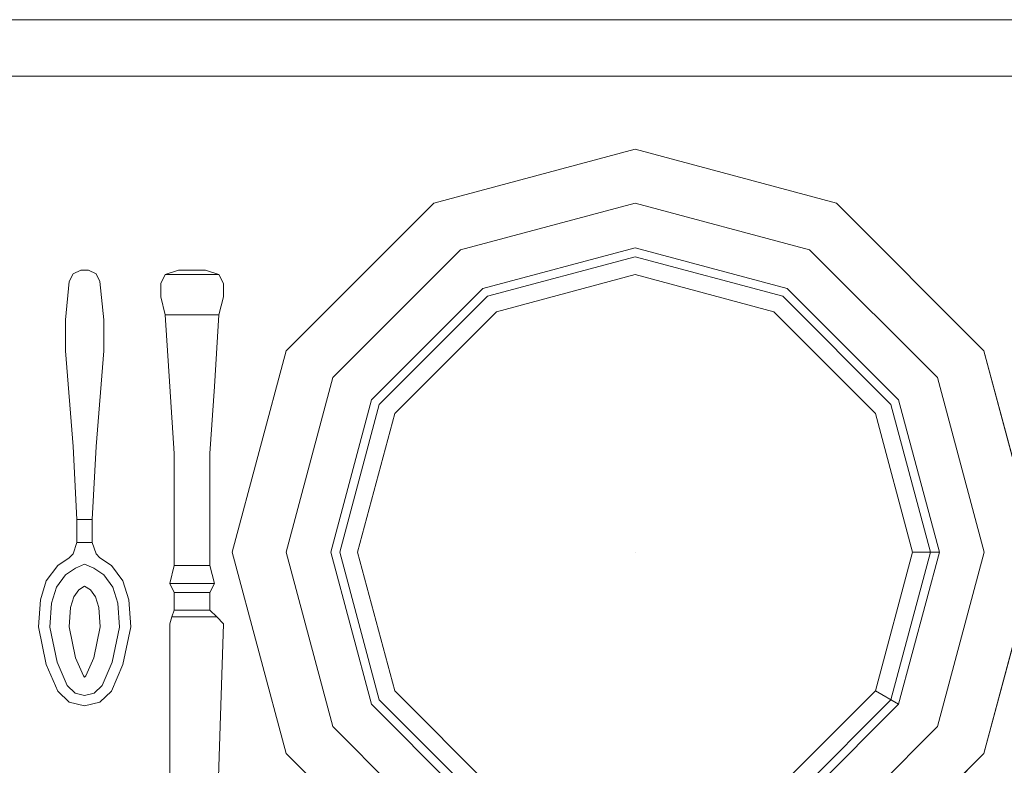
# Model space of a CAD drawing. Units: inches. Extents: x 375 to 1122, y 27 to 1069.
# Tile 54 of 155: x 717.62 to 731.16, y 314.24 to 324.5. Entities that reach past the tile are written whole.
import ezdxf

# ---------------------------------------------------------------- set-up
doc = ezdxf.new("R2010")
doc.units = ezdxf.units.IN
doc.layers.add('Furniture', color=30, linetype='Continuous', lineweight=18)

# ---------------------------------------------------------------- blocks, each defined once
blk = doc.blocks.new('A$C403C54AD')
for p, q in [((0.54488, 0.79569, -0.0006), (0.54488, 1.26108, -0.0006)), ((0.56427, 0.79569, -0.0006), (0.56427, 1.26108, -0.0006))]:
    blk.add_line(p, q)
at = {"linetype": 'ByBlock'}
for points, invisible_edges in [([(0.72796, 1.16691, -0.0197), (0.72796, 1.14844, -0.0197), (0.66793, 1.13235, -0.0197), (0.6587, 1.14835, -0.0197)], 5), ([(0.72796, 1.13305, -0.03355), (0.72796, 1.16691, -0.02431), (0.6587, 1.14835, -0.02431), (0.67563, 1.11902, -0.03355)], 5), ([(0.79723, 1.14835, -0.0197), (0.78799, 1.13235, -0.0197), (0.72796, 1.14844, -0.0197), (0.72796, 1.16691, -0.0197)], 5), ([(0.7803, 1.11902, -0.03355), (0.79723, 1.14835, -0.02431), (0.72796, 1.16691, -0.02431), (0.72796, 1.13305, -0.03355)], 5), ([(0.6587, 1.14835, -0.0197), (0.66793, 1.13235, -0.0197), (0.62399, 1.08841, -0.0197), (0.60799, 1.09765, -0.0197)], 5), ([(0.67563, 1.11902, -0.03355), (0.6587, 1.14835, -0.02431), (0.60799, 1.09765, -0.02431), (0.63732, 1.08071, -0.03355)], 5), ([(0.72796, 1.14844, -0.0197), (0.72796, 1.12997, -0.02585), (0.67717, 1.11636, -0.02585), (0.66793, 1.13235, -0.0197)], 5), ([(0.78799, 1.13235, -0.0197), (0.77876, 1.11636, -0.02585), (0.72796, 1.12997, -0.02585), (0.72796, 1.14844, -0.0197)], 5), ([(0.81861, 1.08071, -0.03355), (0.84793, 1.09765, -0.02431), (0.79723, 1.14835, -0.02431), (0.7803, 1.11902, -0.03355)], 5), ([(0.84793, 1.09765, -0.0197), (0.83194, 1.08841, -0.0197), (0.78799, 1.13235, -0.0197), (0.79723, 1.14835, -0.0197)], 5), ([(0.66793, 1.13235, -0.0197), (0.67717, 1.11636, -0.02585), (0.63999, 1.07918, -0.02585), (0.62399, 1.08841, -0.0197)], 5), ([(0.72796, 1.12381, -0.04278), (0.72796, 1.13305, -0.03355), (0.67563, 1.11902, -0.03355), (0.68025, 1.11103, -0.04278)], 4), ([(0.83194, 1.08841, -0.0197), (0.81594, 1.07918, -0.02585), (0.77876, 1.11636, -0.02585), (0.78799, 1.13235, -0.0197)], 5), ([(0.72796, 1.12997, -0.02585), (0.72796, 1.02838, -0.02585), (0.72796, 1.02838, -0.02585), (0.67717, 1.11636, -0.02585)], 5), ([(0.77876, 1.11636, -0.02585), (0.72796, 1.02838, -0.02585), (0.72796, 1.02838, -0.02585), (0.72796, 1.12997, -0.02585)], 5), ([(0.68025, 1.11103, -0.04278), (0.67563, 1.11902, -0.03355), (0.63732, 1.08071, -0.03355), (0.64532, 1.0761, -0.04278)], 5), ([(0.81061, 1.0761, -0.04278), (0.81861, 1.08071, -0.03355), (0.7803, 1.11902, -0.03355), (0.77568, 1.11103, -0.04278)], 1), ([(0.67717, 1.11636, -0.02585), (0.72796, 1.02838, -0.02585), (0.72796, 1.02838, -0.02585), (0.63999, 1.07918, -0.02585)], 5), ([(0.81594, 1.07918, -0.02585), (0.72796, 1.02838, -0.02585), (0.72796, 1.02838, -0.02585), (0.77876, 1.11636, -0.02585)], 5), ([(0.60799, 1.09765, -0.0197), (0.62399, 1.08841, -0.0197), (0.60791, 1.02838, -0.0197), (0.58944, 1.02838, -0.0197)], 5), ([(0.63732, 1.08071, -0.03355), (0.60799, 1.09765, -0.02431), (0.58944, 1.02838, -0.02431), (0.6233, 1.02838, -0.03355)], 5), ([(0.62399, 1.08841, -0.0197), (0.63999, 1.07918, -0.02585), (0.62638, 1.02838, -0.02585), (0.60791, 1.02838, -0.0197)], 5), ([(0.64532, 1.0761, -0.04278), (0.63732, 1.08071, -0.03355), (0.6233, 1.02838, -0.03355), (0.63253, 1.02838, -0.04278)], 5), ([(0.63999, 1.07918, -0.02585), (0.72796, 1.02838, -0.02585), (0.72796, 1.02838, -0.02585), (0.62638, 1.02838, -0.02585)], 5), ([(0.82955, 1.02838, -0.02585), (0.72796, 1.02838, -0.02585), (0.72796, 1.02838, -0.02585), (0.81594, 1.07918, -0.02585)], 5), ([(0.58944, 1.02838, -0.0197), (0.60791, 1.02838, -0.0197), (0.62399, 0.96835, -0.0197), (0.60799, 0.95912, -0.0197)], 5), ([(0.6233, 1.02838, -0.03355), (0.58944, 1.02838, -0.02431), (0.60799, 0.95912, -0.02431), (0.63732, 0.97605, -0.03355)], 5), ([(0.60791, 1.02838, -0.0197), (0.62638, 1.02838, -0.02585), (0.63999, 0.97759, -0.02585), (0.62399, 0.96835, -0.0197)], 5), ([(0.63253, 1.02838, -0.04278), (0.6233, 1.02838, -0.03355), (0.63732, 0.97605, -0.03355), (0.64532, 0.98067, -0.04278)], 5), ([(0.62638, 1.02838, -0.02585), (0.72796, 1.02838, -0.02585), (0.72796, 1.02838, -0.02585), (0.63999, 0.97759, -0.02585)], 5), ([(0.63999, 0.97759, -0.02585), (0.72796, 1.02838, -0.02585), (0.72796, 1.02838, -0.02585), (0.67717, 0.94041, -0.02585)], 5), ([(0.67717, 0.94041, -0.02585), (0.72796, 1.02838, -0.02585), (0.72796, 1.02838, -0.02585), (0.72796, 0.9268, -0.02585)], 5), ([(0.81594, 0.97759, -0.02585), (0.72796, 1.02838, -0.02585), (0.72796, 1.02838, -0.02585), (0.82955, 1.02838, -0.02585)], 5), ([(0.77876, 0.94041, -0.02585), (0.72796, 1.02838, -0.02585), (0.72796, 1.02838, -0.02585), (0.81594, 0.97759, -0.02585)], 5), ([(0.72796, 0.9268, -0.02585), (0.72796, 1.02838, -0.02585), (0.72796, 1.02838, -0.02585), (0.77876, 0.94041, -0.02585)], 5), ([(0.64532, 0.98067, -0.04278), (0.63732, 0.97605, -0.03355), (0.67563, 0.93774, -0.03355), (0.68025, 0.94574, -0.04278)], 5), ([(0.77568, 0.94574, -0.04278), (0.7803, 0.93774, -0.03355), (0.81861, 0.97605, -0.03355), (0.81061, 0.98067, -0.04278)], 5), ([(0.63732, 0.97605, -0.03355), (0.60799, 0.95912, -0.02431), (0.6587, 0.90841, -0.02431), (0.67563, 0.93774, -0.03355)], 5), ([(0.62399, 0.96835, -0.0197), (0.63999, 0.97759, -0.02585), (0.67717, 0.94041, -0.02585), (0.66793, 0.92441, -0.0197)], 5), ([(0.78799, 0.92441, -0.0197), (0.77876, 0.94041, -0.02585), (0.81594, 0.97759, -0.02585), (0.83194, 0.96835, -0.0197)], 5), ([(0.7803, 0.93774, -0.03355), (0.79723, 0.90841, -0.02431), (0.84793, 0.95912, -0.02431), (0.81861, 0.97605, -0.03355)], 5), ([(0.60799, 0.95912, -0.0197), (0.62399, 0.96835, -0.0197), (0.66793, 0.92441, -0.0197), (0.6587, 0.90841, -0.0197)], 5), ([(0.79723, 0.90841, -0.0197), (0.78799, 0.92441, -0.0197), (0.83194, 0.96835, -0.0197), (0.84793, 0.95912, -0.0197)], 5), ([(0.68025, 0.94574, -0.04278), (0.67563, 0.93774, -0.03355), (0.72796, 0.92372, -0.03355), (0.72796, 0.93295, -0.04278)], 5), ([(0.72796, 0.93295, -0.04278), (0.72796, 0.92372, -0.03355), (0.7803, 0.93774, -0.03355), (0.77568, 0.94574, -0.04278)], 5), ([(0.66793, 0.92441, -0.0197), (0.67717, 0.94041, -0.02585), (0.72796, 0.9268, -0.02585), (0.72796, 0.90833, -0.0197)], 5), ([(0.72796, 0.90833, -0.0197), (0.72796, 0.9268, -0.02585), (0.77876, 0.94041, -0.02585), (0.78799, 0.92441, -0.0197)], 5), ([(0.67563, 0.93774, -0.03355), (0.6587, 0.90841, -0.02431), (0.72796, 0.88985, -0.02431), (0.72796, 0.92372, -0.03355)], 5), ([(0.72796, 0.92372, -0.03355), (0.72796, 0.88985, -0.02431), (0.79723, 0.90841, -0.02431), (0.7803, 0.93774, -0.03355)], 5), ([(0.6587, 0.90841, -0.0197), (0.66793, 0.92441, -0.0197), (0.72796, 0.90833, -0.0197), (0.72796, 0.88985, -0.0197)], 5), ([(0.72796, 0.88985, -0.0197), (0.72796, 0.90833, -0.0197), (0.78799, 0.92441, -0.0197), (0.79723, 0.90841, -0.0197)], 5)]:
    blk.add_3dface(points, dxfattribs=dict(at, invisible_edges=invisible_edges))
for points in [[(0.72796, 1.16691, -0.02431), (0.72796, 1.16691, -0.0197), (0.6587, 1.14835, -0.0197), (0.6587, 1.14835, -0.02431)], [(0.79723, 1.14835, -0.02431), (0.79723, 1.14835, -0.0197), (0.72796, 1.16691, -0.0197), (0.72796, 1.16691, -0.02431)], [(0.6587, 1.14835, -0.02431), (0.6587, 1.14835, -0.0197), (0.60799, 1.09765, -0.0197), (0.60799, 1.09765, -0.02431)], [(0.84793, 1.09765, -0.02431), (0.84793, 1.09765, -0.0197), (0.79723, 1.14835, -0.0197), (0.79723, 1.14835, -0.02431)], [(0.77568, 1.11103, -0.04278), (0.7803, 1.11902, -0.03355), (0.72796, 1.13305, -0.03355), (0.72796, 1.12381, -0.04278)], [(0.60799, 1.09765, -0.02431), (0.60799, 1.09765, -0.0197), (0.58944, 1.02838, -0.0197), (0.58944, 1.02838, -0.02431)], [(0.58944, 1.02838, -0.02431), (0.58944, 1.02838, -0.0197), (0.60799, 0.95912, -0.0197), (0.60799, 0.95912, -0.02431)], [(0.60799, 0.95912, -0.02431), (0.60799, 0.95912, -0.0197), (0.6587, 0.90841, -0.0197), (0.6587, 0.90841, -0.02431)], [(0.79723, 0.90841, -0.02431), (0.79723, 0.90841, -0.0197), (0.84793, 0.95912, -0.0197), (0.84793, 0.95912, -0.02431)], [(0.6587, 0.90841, -0.02431), (0.6587, 0.90841, -0.0197), (0.72796, 0.88985, -0.0197), (0.72796, 0.88985, -0.02431)], [(0.72796, 0.88985, -0.02431), (0.72796, 0.88985, -0.0197), (0.79723, 0.90841, -0.0197), (0.79723, 0.90841, -0.02431)]]:
    blk.add_3dface(points, dxfattribs=at)
for points in [[(0.63253, 0.88524, -0.03355), (0.63253, 0.86677, -0.03355), (0.63099, 0.87138, -0.03663), (0.63099, 0.88062, -0.03663)], [(0.63253, 0.88524, -0.03355), (0.63253, 0.88524, -0.03971), (0.63099, 0.88062, -0.03663)], [(0.63253, 0.88524, -0.03971), (0.63253, 0.86677, -0.03971), (0.63099, 0.87138, -0.03663), (0.63099, 0.88062, -0.03663)], [(0.63561, 0.88678, -0.04124), (0.63561, 0.88678, -0.03201), (0.63253, 0.88524, -0.03355), (0.63253, 0.88524, -0.03971)], [(0.64023, 0.88678, -0.03047), (0.64023, 0.88678, -0.04278), (0.63561, 0.88678, -0.04124), (0.63561, 0.88678, -0.03201)], [(0.64639, 0.88524, -0.04124), (0.64639, 0.88524, -0.03201), (0.64023, 0.88678, -0.03047), (0.64023, 0.88678, -0.04278)], [(0.67101, 0.8837, -0.03047), (0.67101, 0.8837, -0.04278), (0.64639, 0.88524, -0.04124), (0.64639, 0.88524, -0.03201)], [(0.75028, 0.88447, -0.03509), (0.75028, 0.86908, -0.03509), (0.74797, 0.86985, -0.03201), (0.74797, 0.88216, -0.03201)], [(0.75028, 0.88447, -0.03817), (0.75028, 0.86908, -0.03817), (0.74797, 0.86985, -0.04124), (0.74797, 0.88216, -0.04124)], [(0.6941, 0.88216, -0.04278), (0.6941, 0.88216, -0.03047), (0.67101, 0.8837, -0.03047), (0.67101, 0.8837, -0.04278)], [(0.73258, 0.88216, -0.03201), (0.73258, 0.88216, -0.04124), (0.6941, 0.88216, -0.04278), (0.6941, 0.88216, -0.03047)], [(0.73874, 0.86831, -0.03047), (0.73874, 0.8837, -0.03047), (0.73258, 0.88216, -0.03201), (0.73258, 0.86985, -0.03201)], [(0.73874, 0.86831, -0.04278), (0.73874, 0.8837, -0.04278), (0.73258, 0.88216, -0.04124), (0.73258, 0.86985, -0.04124)], [(0.73874, 0.8837, -0.04278), (0.73874, 0.8837, -0.03047), (0.73258, 0.88216, -0.03201), (0.73258, 0.88216, -0.04124)], [(0.74182, 0.88216, -0.03201), (0.74182, 0.86985, -0.03201), (0.73874, 0.86831, -0.03047), (0.73874, 0.8837, -0.03047)], [(0.74182, 0.88216, -0.04124), (0.74182, 0.86985, -0.04124), (0.73874, 0.86831, -0.04278), (0.73874, 0.8837, -0.04278)], [(0.74182, 0.88216, -0.03201), (0.74182, 0.88216, -0.04124), (0.73874, 0.8837, -0.04278), (0.73874, 0.8837, -0.03047)], [(0.74797, 0.86985, -0.03201), (0.74797, 0.88216, -0.03201), (0.74182, 0.88216, -0.03201), (0.74182, 0.86985, -0.03201)], [(0.74797, 0.86985, -0.04124), (0.74797, 0.88216, -0.04124), (0.74182, 0.88216, -0.04124), (0.74182, 0.86985, -0.04124)], [(0.63099, 0.87138, -0.03663), (0.63099, 0.87138, -0.03663), (0.63253, 0.86677, -0.03355), (0.63253, 0.86677, -0.03971)], [(0.64639, 0.86677, -0.03201), (0.64639, 0.86677, -0.04124), (0.67101, 0.86831, -0.04278), (0.67101, 0.86831, -0.03047)], [(0.67101, 0.86831, -0.04278), (0.67101, 0.86831, -0.03047), (0.6941, 0.86985, -0.03047), (0.6941, 0.86985, -0.04278)], [(0.6941, 0.86985, -0.03047), (0.6941, 0.86985, -0.04278), (0.73258, 0.86985, -0.04124), (0.73258, 0.86985, -0.03201)], [(0.73258, 0.86985, -0.04124), (0.73258, 0.86985, -0.03201), (0.73874, 0.86831, -0.03047), (0.73874, 0.86831, -0.04278)], [(0.73874, 0.86831, -0.03047), (0.73874, 0.86831, -0.04278), (0.74182, 0.86985, -0.04124), (0.74182, 0.86985, -0.03201)], [(0.63253, 0.86677, -0.03355), (0.63253, 0.86677, -0.03971), (0.63561, 0.86523, -0.04124), (0.63561, 0.86523, -0.03201)], [(0.63561, 0.86523, -0.03201), (0.63561, 0.86523, -0.04124), (0.64023, 0.86523, -0.04278), (0.64023, 0.86523, -0.03047)], [(0.64023, 0.86523, -0.04278), (0.64023, 0.86523, -0.03047), (0.64639, 0.86677, -0.03201), (0.64639, 0.86677, -0.04124)], [(0.74443, 0.85423, -0.03727), (0.74443, 0.85423, -0.03595), (0.73783, 0.85225, -0.03635), (0.73783, 0.85225, -0.03767)], [(0.75364, 0.85489, -0.0364), (0.75364, 0.85489, -0.03508), (0.74443, 0.85423, -0.03595), (0.74443, 0.85423, -0.03727)], [(0.76668, 0.85225, -0.03304), (0.76668, 0.85225, -0.03436), (0.75364, 0.85489, -0.0364), (0.75364, 0.85489, -0.03508)], [(0.73783, 0.85225, -0.03635), (0.73783, 0.85225, -0.03767), (0.73257, 0.8483, -0.03815), (0.73257, 0.8483, -0.03683)], [(0.77574, 0.8483, -0.03252), (0.77574, 0.8483, -0.03121), (0.76668, 0.85225, -0.03304), (0.76668, 0.85225, -0.03436)], [(0.73257, 0.8483, -0.03815), (0.73257, 0.8483, -0.03683), (0.72996, 0.84434, -0.03721), (0.72996, 0.84434, -0.03936)], [(0.77958, 0.84434, -0.03012), (0.77958, 0.84434, -0.03144), (0.77574, 0.8483, -0.03252), (0.77574, 0.8483, -0.03121)], [(0.63495, 0.84434, -0.03878), (0.63495, 0.84434, -0.04275), (0.63231, 0.84302, -0.04254), (0.63231, 0.84302, -0.03857)], [(0.64814, 0.84566, -0.04278), (0.64814, 0.84566, -0.03881), (0.63495, 0.84434, -0.03878), (0.63495, 0.84434, -0.04275)], [(0.6587, 0.84566, -0.03853), (0.6587, 0.84566, -0.0425), (0.64814, 0.84566, -0.04278), (0.64814, 0.84566, -0.03881)], [(0.78089, 0.83906, -0.03125), (0.78089, 0.83906, -0.02993), (0.77958, 0.84434, -0.03012), (0.77958, 0.84434, -0.03144)], [(0.63231, 0.84302, -0.04254), (0.63231, 0.84302, -0.03857), (0.63099, 0.84038, -0.03871), (0.63099, 0.84038, -0.04225)], [(0.63099, 0.84038, -0.03871), (0.63099, 0.84038, -0.04225), (0.63099, 0.83774, -0.04225), (0.63099, 0.83774, -0.03871)], [(0.71675, 0.8417, -0.03621), (0.71675, 0.83642, -0.03621), (0.72466, 0.83642, -0.03684), (0.72466, 0.8417, -0.03684)], [(0.71675, 0.8417, -0.03399), (0.71675, 0.83642, -0.03399), (0.72466, 0.83642, -0.03462), (0.72466, 0.8417, -0.03462)], [(0.63099, 0.83774, -0.04225), (0.63099, 0.83774, -0.03871), (0.63231, 0.8351, -0.03857), (0.63231, 0.8351, -0.04254)], [(0.77958, 0.83378, -0.03012), (0.77958, 0.83378, -0.03144), (0.78089, 0.83906, -0.03125), (0.78089, 0.83906, -0.02993)], [(0.63231, 0.8351, -0.03857), (0.63231, 0.8351, -0.04254), (0.63495, 0.83378, -0.04275), (0.63495, 0.83378, -0.03878)], [(0.63495, 0.83378, -0.04275), (0.63495, 0.83378, -0.03878), (0.64814, 0.83247, -0.03881), (0.64814, 0.83247, -0.04278)], [(0.72996, 0.83378, -0.03936), (0.72996, 0.83378, -0.03721), (0.73257, 0.82983, -0.03683), (0.73257, 0.82983, -0.03815)], [(0.77574, 0.82983, -0.03252), (0.77574, 0.82983, -0.03121), (0.77958, 0.83378, -0.03012), (0.77958, 0.83378, -0.03144)], [(0.64814, 0.83247, -0.03881), (0.64814, 0.83247, -0.04278), (0.6587, 0.83247, -0.0425), (0.6587, 0.83247, -0.03853)], [(0.73257, 0.82983, -0.03683), (0.73257, 0.82983, -0.03815), (0.73783, 0.82587, -0.03767), (0.73783, 0.82587, -0.03635)], [(0.76668, 0.82587, -0.03304), (0.76668, 0.82587, -0.03436), (0.77574, 0.82983, -0.03252), (0.77574, 0.82983, -0.03121)], [(0.73783, 0.82587, -0.03767), (0.73783, 0.82587, -0.03635), (0.74443, 0.82389, -0.03595), (0.74443, 0.82389, -0.03727)], [(0.74443, 0.82389, -0.03595), (0.74443, 0.82389, -0.03727), (0.75364, 0.82323, -0.0364), (0.75364, 0.82323, -0.03508)], [(0.75364, 0.82323, -0.0364), (0.75364, 0.82323, -0.03508), (0.76668, 0.82587, -0.03304), (0.76668, 0.82587, -0.03436)]]:
    blk.add_3dface(points)
for points, invisible_edges in [([(0.63561, 0.86523, -0.03201), (0.63561, 0.88678, -0.03201), (0.63253, 0.88524, -0.03355), (0.63253, 0.86677, -0.03355)], 1), ([(0.63561, 0.86523, -0.04124), (0.63561, 0.88678, -0.04124), (0.63253, 0.88524, -0.03971), (0.63253, 0.86677, -0.03971)], 1), ([(0.64023, 0.88678, -0.03047), (0.64023, 0.86523, -0.03047), (0.63561, 0.86523, -0.03201), (0.63561, 0.88678, -0.03201)], 5), ([(0.64023, 0.88678, -0.04278), (0.64023, 0.86523, -0.04278), (0.63561, 0.86523, -0.04124), (0.63561, 0.88678, -0.04124)], 5), ([(0.64639, 0.86677, -0.03201), (0.64639, 0.88524, -0.03201), (0.64023, 0.88678, -0.03047), (0.64023, 0.86523, -0.03047)], 4), ([(0.64639, 0.86677, -0.04124), (0.64639, 0.88524, -0.04124), (0.64023, 0.88678, -0.04278), (0.64023, 0.86523, -0.04278)], 4), ([(0.67101, 0.8837, -0.03047), (0.67101, 0.86831, -0.03047), (0.64639, 0.86677, -0.03201), (0.64639, 0.88524, -0.03201)], 1), ([(0.67101, 0.8837, -0.04278), (0.67101, 0.86831, -0.04278), (0.64639, 0.86677, -0.04124), (0.64639, 0.88524, -0.04124)], 1), ([(0.75028, 0.88447, -0.03509), (0.75028, 0.88447, -0.03817), (0.74797, 0.88216, -0.04124), (0.74797, 0.88216, -0.03201)], 5), ([(0.75259, 0.88678, -0.03586), (0.75259, 0.86831, -0.03586), (0.75028, 0.86908, -0.03509), (0.75028, 0.88447, -0.03509)], 1), ([(0.75259, 0.88678, -0.0374), (0.75259, 0.86831, -0.0374), (0.75028, 0.86908, -0.03817), (0.75028, 0.88447, -0.03817)], 1), ([(0.75259, 0.88678, -0.0374), (0.75259, 0.88678, -0.03586), (0.75028, 0.88447, -0.03509), (0.75028, 0.88447, -0.03817)], 5), ([(0.81108, 0.86831, -0.03586), (0.84956, 0.8837, -0.03586), (0.75259, 0.88678, -0.03586), (0.75259, 0.86831, -0.03586)], 5), ([(0.81108, 0.86831, -0.0374), (0.84956, 0.8837, -0.0374), (0.75259, 0.88678, -0.0374), (0.75259, 0.86831, -0.0374)], 5), ([(0.84956, 0.8837, -0.0374), (0.84956, 0.8837, -0.03586), (0.75259, 0.88678, -0.03586), (0.75259, 0.88678, -0.0374)], 5), ([(0.6941, 0.86985, -0.03047), (0.6941, 0.88216, -0.03047), (0.67101, 0.8837, -0.03047), (0.67101, 0.86831, -0.03047)], 5), ([(0.6941, 0.86985, -0.04278), (0.6941, 0.88216, -0.04278), (0.67101, 0.8837, -0.04278), (0.67101, 0.86831, -0.04278)], 5), ([(0.73258, 0.88216, -0.03201), (0.73258, 0.86985, -0.03201), (0.6941, 0.86985, -0.03047), (0.6941, 0.88216, -0.03047)], 4), ([(0.73258, 0.88216, -0.04124), (0.73258, 0.86985, -0.04124), (0.6941, 0.86985, -0.04278), (0.6941, 0.88216, -0.04278)], 4), ([(0.74797, 0.88216, -0.04124), (0.74797, 0.88216, -0.03201), (0.74182, 0.88216, -0.03201), (0.74182, 0.88216, -0.04124)], 1), ([(0.74182, 0.86985, -0.04124), (0.74182, 0.86985, -0.03201), (0.74797, 0.86985, -0.03201), (0.74797, 0.86985, -0.04124)], 4), ([(0.74797, 0.86985, -0.03201), (0.74797, 0.86985, -0.04124), (0.75028, 0.86908, -0.03817), (0.75028, 0.86908, -0.03509)], 5), ([(0.75028, 0.86908, -0.03817), (0.75028, 0.86908, -0.03509), (0.75259, 0.86831, -0.03586), (0.75259, 0.86831, -0.0374)], 5), ([(0.75259, 0.86831, -0.03586), (0.75259, 0.86831, -0.0374), (0.81108, 0.86831, -0.0374), (0.81108, 0.86831, -0.03586)], 5), ([(0.73998, 0.84876, -0.03894), (0.73783, 0.85225, -0.03635), (0.74443, 0.85423, -0.03595), (0.7455, 0.85042, -0.03843)], 5), ([(0.73998, 0.84876, -0.04026), (0.73783, 0.85225, -0.03767), (0.74443, 0.85423, -0.03727), (0.7455, 0.85042, -0.03975)], 5), ([(0.74443, 0.85423, -0.03595), (0.7455, 0.85042, -0.03843), (0.75374, 0.85101, -0.03754), (0.75364, 0.85489, -0.03508)], 5), ([(0.74443, 0.85423, -0.03727), (0.7455, 0.85042, -0.03975), (0.75374, 0.85101, -0.03886), (0.75364, 0.85489, -0.0364)], 5), ([(0.75374, 0.85101, -0.03886), (0.75364, 0.85489, -0.0364), (0.76668, 0.85225, -0.03436), (0.76587, 0.84855, -0.03687)], 5), ([(0.75374, 0.85101, -0.03754), (0.75364, 0.85489, -0.03508), (0.76668, 0.85225, -0.03304), (0.76587, 0.84855, -0.03555)], 5), ([(0.73257, 0.8483, -0.03815), (0.73576, 0.84561, -0.04043), (0.73998, 0.84876, -0.04026), (0.73783, 0.85225, -0.03767)], 5), ([(0.73257, 0.8483, -0.03683), (0.73576, 0.84561, -0.03911), (0.73998, 0.84876, -0.03894), (0.73783, 0.85225, -0.03635)], 5), ([(0.74707, 0.84391, -0.04103), (0.7455, 0.85042, -0.03843), (0.73998, 0.84876, -0.03894), (0.74335, 0.84279, -0.04126)], 5), ([(0.75374, 0.85101, -0.03886), (0.75368, 0.84439, -0.0414), (0.74707, 0.84391, -0.04234), (0.7455, 0.85042, -0.03975)], 5), ([(0.75374, 0.85101, -0.03754), (0.75368, 0.84439, -0.04008), (0.74707, 0.84391, -0.04103), (0.7455, 0.85042, -0.03843)], 5), ([(0.76429, 0.84224, -0.03837), (0.76587, 0.84855, -0.03555), (0.75374, 0.85101, -0.03754), (0.75368, 0.84439, -0.04008)], 5), ([(0.76429, 0.84224, -0.03969), (0.76587, 0.84855, -0.03687), (0.75374, 0.85101, -0.03886), (0.75368, 0.84439, -0.0414)], 5), ([(0.76668, 0.85225, -0.03436), (0.76587, 0.84855, -0.03687), (0.7739, 0.84505, -0.03516), (0.77574, 0.8483, -0.03252)], 5), ([(0.76668, 0.85225, -0.03304), (0.76587, 0.84855, -0.03555), (0.7739, 0.84505, -0.03385), (0.77574, 0.8483, -0.03121)], 5), ([(0.73347, 0.8422, -0.03912), (0.72996, 0.84434, -0.03721), (0.73257, 0.8483, -0.03683), (0.73576, 0.84561, -0.03911)], 5), ([(0.73998, 0.84876, -0.04026), (0.74335, 0.84279, -0.04258), (0.74098, 0.84102, -0.04267), (0.73576, 0.84561, -0.04043)], 5), ([(0.73998, 0.84876, -0.03894), (0.74335, 0.84279, -0.04126), (0.74098, 0.84102, -0.04136), (0.73576, 0.84561, -0.03911)], 5), ([(0.7739, 0.84505, -0.03516), (0.77052, 0.8395, -0.03806), (0.76429, 0.84224, -0.03969), (0.76587, 0.84855, -0.03687)], 5), ([(0.7739, 0.84505, -0.03385), (0.77052, 0.8395, -0.03674), (0.76429, 0.84224, -0.03837), (0.76587, 0.84855, -0.03555)], 5), ([(0.7739, 0.84505, -0.03516), (0.77574, 0.8483, -0.03252), (0.77958, 0.84434, -0.03144), (0.77652, 0.84237, -0.03461)], 5), ([(0.7739, 0.84505, -0.03385), (0.77574, 0.8483, -0.03121), (0.77958, 0.84434, -0.03012), (0.77652, 0.84237, -0.03329)], 5), ([(0.63231, 0.8351, -0.03857), (0.63231, 0.84302, -0.03857), (0.63495, 0.84434, -0.03878), (0.63495, 0.83378, -0.03878)], 5), ([(0.63231, 0.8351, -0.04254), (0.63231, 0.84302, -0.04254), (0.63495, 0.84434, -0.04275), (0.63495, 0.83378, -0.04275)], 5), ([(0.63495, 0.84434, -0.03878), (0.63495, 0.83378, -0.03878), (0.64814, 0.83247, -0.03881), (0.64814, 0.84566, -0.03881)], 5), ([(0.63495, 0.84434, -0.04275), (0.63495, 0.83378, -0.04275), (0.64814, 0.83247, -0.04278), (0.64814, 0.84566, -0.04278)], 5), ([(0.64814, 0.83247, -0.03881), (0.64814, 0.84566, -0.03881), (0.6587, 0.84566, -0.03853), (0.6587, 0.83247, -0.03853)], 5), ([(0.64814, 0.83247, -0.04278), (0.64814, 0.84566, -0.04278), (0.6587, 0.84566, -0.0425), (0.6587, 0.83247, -0.0425)], 5), ([(0.6587, 0.84566, -0.0425), (0.6587, 0.83247, -0.0425), (0.69168, 0.8351, -0.03912), (0.69168, 0.84302, -0.03912)], 5), ([(0.69168, 0.84302, -0.03912), (0.69168, 0.84302, -0.03648), (0.6587, 0.84566, -0.03853), (0.6587, 0.84566, -0.0425)], 1), ([(0.6587, 0.84566, -0.03853), (0.6587, 0.83247, -0.03853), (0.69168, 0.8351, -0.03648), (0.69168, 0.84302, -0.03648)], 5), ([(0.72862, 0.84302, -0.03647), (0.72862, 0.8351, -0.03647), (0.72996, 0.83378, -0.03721), (0.72996, 0.84434, -0.03721)], 5), ([(0.72862, 0.84302, -0.03856), (0.72862, 0.8351, -0.03856), (0.72996, 0.83378, -0.03936), (0.72996, 0.84434, -0.03936)], 5), ([(0.72862, 0.84302, -0.03647), (0.72862, 0.84302, -0.03856), (0.72996, 0.84434, -0.03936), (0.72996, 0.84434, -0.03721)], 1), ([(0.72996, 0.84434, -0.03936), (0.72996, 0.83906, -0.03936), (0.73211, 0.83906, -0.04026), (0.73347, 0.8422, -0.04044)], 11), ([(0.72996, 0.84434, -0.03721), (0.72996, 0.83906, -0.03721), (0.73211, 0.83906, -0.03894), (0.73347, 0.8422, -0.03912)], 11), ([(0.74098, 0.84102, -0.04267), (0.73576, 0.84561, -0.04043), (0.73347, 0.8422, -0.04044), (0.73963, 0.83906, -0.04247)], 5), ([(0.74098, 0.84102, -0.04136), (0.73576, 0.84561, -0.03911), (0.73347, 0.8422, -0.03912), (0.73963, 0.83906, -0.04116)], 5), ([(0.74707, 0.83421, -0.04234), (0.74707, 0.84391, -0.04234), (0.74335, 0.84279, -0.04258), (0.74335, 0.83533, -0.04258)], 5), ([(0.74707, 0.83421, -0.04103), (0.74707, 0.84391, -0.04103), (0.74335, 0.84279, -0.04126), (0.74335, 0.83533, -0.04126)], 5), ([(0.75368, 0.84439, -0.0414), (0.75368, 0.83374, -0.0414), (0.74707, 0.83421, -0.04234), (0.74707, 0.84391, -0.04234)], 5), ([(0.75368, 0.84439, -0.04008), (0.75368, 0.83374, -0.04008), (0.74707, 0.83421, -0.04103), (0.74707, 0.84391, -0.04103)], 5), ([(0.76429, 0.83589, -0.03837), (0.76429, 0.84224, -0.03837), (0.75368, 0.84439, -0.04008), (0.75368, 0.83374, -0.04008)], 5), ([(0.76429, 0.83589, -0.03969), (0.76429, 0.84224, -0.03969), (0.75368, 0.84439, -0.0414), (0.75368, 0.83374, -0.0414)], 5), ([(0.77052, 0.8395, -0.03674), (0.77652, 0.84237, -0.03329), (0.7739, 0.84505, -0.03385), (0.77052, 0.8395, -0.03674)], 5), ([(0.77052, 0.8395, -0.03806), (0.77652, 0.84237, -0.03461), (0.7739, 0.84505, -0.03516), (0.77052, 0.8395, -0.03806)], 5), ([(0.77958, 0.84434, -0.03144), (0.77652, 0.84237, -0.03461), (0.77733, 0.83906, -0.03442), (0.78089, 0.83906, -0.03125)], 5), ([(0.77958, 0.84434, -0.03012), (0.77652, 0.84237, -0.03329), (0.77733, 0.83906, -0.0331), (0.78089, 0.83906, -0.02993)], 5), ([(0.63099, 0.84038, -0.03871), (0.63099, 0.83774, -0.03871), (0.63231, 0.8351, -0.03857), (0.63231, 0.84302, -0.03857)], 4), ([(0.63099, 0.84038, -0.04225), (0.63099, 0.83774, -0.04225), (0.63231, 0.8351, -0.04254), (0.63231, 0.84302, -0.04254)], 4), ([(0.69168, 0.8351, -0.03648), (0.69168, 0.84302, -0.03648), (0.71675, 0.8417, -0.03399), (0.71675, 0.83642, -0.03399)], 1), ([(0.71675, 0.8417, -0.03399), (0.71675, 0.8417, -0.03621), (0.69168, 0.84302, -0.03912), (0.69168, 0.84302, -0.03648)], 5), ([(0.69168, 0.8351, -0.03912), (0.69168, 0.84302, -0.03912), (0.71675, 0.8417, -0.03621), (0.71675, 0.83642, -0.03621)], 1), ([(0.72466, 0.8417, -0.03684), (0.72466, 0.8417, -0.03462), (0.71675, 0.8417, -0.03399), (0.71675, 0.8417, -0.03621)], 5), ([(0.72466, 0.83642, -0.03462), (0.72466, 0.8417, -0.03462), (0.72862, 0.84302, -0.03647), (0.72862, 0.8351, -0.03647)], 4), ([(0.72466, 0.8417, -0.03684), (0.72466, 0.8417, -0.03462), (0.72862, 0.84302, -0.03647), (0.72862, 0.84302, -0.03856)], 5), ([(0.72466, 0.83642, -0.03684), (0.72466, 0.8417, -0.03684), (0.72862, 0.84302, -0.03856), (0.72862, 0.8351, -0.03856)], 4), ([(0.73347, 0.8422, -0.04044), (0.73963, 0.83906, -0.04247), (0.73963, 0.83906, -0.04247), (0.73211, 0.83906, -0.04026)], 5), ([(0.73347, 0.8422, -0.03912), (0.73963, 0.83906, -0.04116), (0.73963, 0.83906, -0.04116), (0.73211, 0.83906, -0.03894)], 5), ([(0.74098, 0.8371, -0.04267), (0.74098, 0.84102, -0.04267), (0.73963, 0.83906, -0.04247)], 1), ([(0.74098, 0.8371, -0.04136), (0.74098, 0.84102, -0.04136), (0.73963, 0.83906, -0.04116)], 1), ([(0.74335, 0.84279, -0.04258), (0.74335, 0.83533, -0.04258), (0.74098, 0.8371, -0.04267), (0.74098, 0.84102, -0.04267)], 5), ([(0.74335, 0.84279, -0.04126), (0.74335, 0.83533, -0.04126), (0.74098, 0.8371, -0.04136), (0.74098, 0.84102, -0.04136)], 5), ([(0.77052, 0.8395, -0.03806), (0.77052, 0.83862, -0.03806), (0.76429, 0.83589, -0.03969), (0.76429, 0.84224, -0.03969)], 5), ([(0.77052, 0.8395, -0.03674), (0.77052, 0.83862, -0.03674), (0.76429, 0.83589, -0.03837), (0.76429, 0.84224, -0.03837)], 5), ([(0.77733, 0.83906, -0.0331), (0.77094, 0.83906, -0.0366), (0.77052, 0.8395, -0.03674), (0.77652, 0.84237, -0.03329)], 5), ([(0.77733, 0.83906, -0.03442), (0.77094, 0.83906, -0.03792), (0.77052, 0.8395, -0.03806), (0.77652, 0.84237, -0.03461)], 5), ([(0.72996, 0.83378, -0.03936), (0.72996, 0.83906, -0.03936), (0.73211, 0.83906, -0.04026), (0.73347, 0.83592, -0.04044)], 11), ([(0.72996, 0.83378, -0.03721), (0.72996, 0.83906, -0.03721), (0.73211, 0.83906, -0.03894), (0.73347, 0.83592, -0.03912)], 11), ([(0.73347, 0.83592, -0.04044), (0.73963, 0.83906, -0.04247), (0.73963, 0.83906, -0.04247), (0.73211, 0.83906, -0.04026)], 5), ([(0.73347, 0.83592, -0.03912), (0.73963, 0.83906, -0.04116), (0.73963, 0.83906, -0.04116), (0.73211, 0.83906, -0.03894)], 5), ([(0.74098, 0.8371, -0.04267), (0.73576, 0.83251, -0.04043), (0.73347, 0.83592, -0.04044), (0.73963, 0.83906, -0.04247)], 5), ([(0.74098, 0.8371, -0.04136), (0.73576, 0.83251, -0.03911), (0.73347, 0.83592, -0.03912), (0.73963, 0.83906, -0.04116)], 5), ([(0.73998, 0.82936, -0.04026), (0.74335, 0.83533, -0.04258), (0.74098, 0.8371, -0.04267), (0.73576, 0.83251, -0.04043)], 5), ([(0.73998, 0.82936, -0.03894), (0.74335, 0.83533, -0.04126), (0.74098, 0.8371, -0.04136), (0.73576, 0.83251, -0.03911)], 5), ([(0.7739, 0.83308, -0.03516), (0.77052, 0.83862, -0.03806), (0.76429, 0.83589, -0.03969), (0.76587, 0.82957, -0.03687)], 5), ([(0.7739, 0.83308, -0.03385), (0.77052, 0.83862, -0.03674), (0.76429, 0.83589, -0.03837), (0.76587, 0.82957, -0.03555)], 5), ([(0.77094, 0.83906, -0.0366), (0.77052, 0.83862, -0.03674), (0.77052, 0.8395, -0.03674), (0.77094, 0.83906, -0.0366)], 2), ([(0.77094, 0.83906, -0.03792), (0.77052, 0.83862, -0.03806), (0.77052, 0.8395, -0.03806), (0.77094, 0.83906, -0.03792)], 2), ([(0.77733, 0.83906, -0.0331), (0.77094, 0.83906, -0.0366), (0.77052, 0.83862, -0.03674), (0.77652, 0.83575, -0.03329)], 5), ([(0.77733, 0.83906, -0.03442), (0.77094, 0.83906, -0.03792), (0.77052, 0.83862, -0.03806), (0.77652, 0.83575, -0.03461)], 5), ([(0.77052, 0.83862, -0.03674), (0.77652, 0.83575, -0.03329), (0.7739, 0.83308, -0.03385), (0.77052, 0.83862, -0.03674)], 5), ([(0.77052, 0.83862, -0.03806), (0.77652, 0.83575, -0.03461), (0.7739, 0.83308, -0.03516), (0.77052, 0.83862, -0.03806)], 5), ([(0.77958, 0.83378, -0.03144), (0.77652, 0.83575, -0.03461), (0.77733, 0.83906, -0.03442), (0.78089, 0.83906, -0.03125)], 5), ([(0.77958, 0.83378, -0.03012), (0.77652, 0.83575, -0.03329), (0.77733, 0.83906, -0.0331), (0.78089, 0.83906, -0.02993)], 5), ([(0.6587, 0.83247, -0.0425), (0.6587, 0.83247, -0.03853), (0.69168, 0.8351, -0.03648), (0.69168, 0.8351, -0.03912)], 4), ([(0.69168, 0.8351, -0.03648), (0.69168, 0.8351, -0.03912), (0.71675, 0.83642, -0.03621), (0.71675, 0.83642, -0.03399)], 5), ([(0.71675, 0.83642, -0.03621), (0.71675, 0.83642, -0.03399), (0.72466, 0.83642, -0.03462), (0.72466, 0.83642, -0.03684)], 5), ([(0.72466, 0.83642, -0.03462), (0.72466, 0.83642, -0.03684), (0.72862, 0.8351, -0.03856), (0.72862, 0.8351, -0.03647)], 5), ([(0.72862, 0.8351, -0.03856), (0.72862, 0.8351, -0.03647), (0.72996, 0.83378, -0.03721), (0.72996, 0.83378, -0.03936)], 1), ([(0.73347, 0.83592, -0.04044), (0.72996, 0.83378, -0.03936), (0.73257, 0.82983, -0.03815), (0.73576, 0.83251, -0.04043)], 5), ([(0.73347, 0.83592, -0.03912), (0.72996, 0.83378, -0.03721), (0.73257, 0.82983, -0.03683), (0.73576, 0.83251, -0.03911)], 5), ([(0.74707, 0.83421, -0.04234), (0.7455, 0.8277, -0.03975), (0.73998, 0.82936, -0.04026), (0.74335, 0.83533, -0.04258)], 5), ([(0.74707, 0.83421, -0.04103), (0.7455, 0.8277, -0.03843), (0.73998, 0.82936, -0.03894), (0.74335, 0.83533, -0.04126)], 5), ([(0.75374, 0.82711, -0.03886), (0.75368, 0.83374, -0.0414), (0.74707, 0.83421, -0.04234), (0.7455, 0.8277, -0.03975)], 5), ([(0.75374, 0.82711, -0.03754), (0.75368, 0.83374, -0.04008), (0.74707, 0.83421, -0.04103), (0.7455, 0.8277, -0.03843)], 5), ([(0.76429, 0.83589, -0.03837), (0.76587, 0.82957, -0.03555), (0.75374, 0.82711, -0.03754), (0.75368, 0.83374, -0.04008)], 5), ([(0.76429, 0.83589, -0.03969), (0.76587, 0.82957, -0.03687), (0.75374, 0.82711, -0.03886), (0.75368, 0.83374, -0.0414)], 5), ([(0.76668, 0.82587, -0.03436), (0.76587, 0.82957, -0.03687), (0.7739, 0.83308, -0.03516), (0.77574, 0.82983, -0.03252)], 5), ([(0.76668, 0.82587, -0.03304), (0.76587, 0.82957, -0.03555), (0.7739, 0.83308, -0.03385), (0.77574, 0.82983, -0.03121)], 5), ([(0.7739, 0.83308, -0.03516), (0.77574, 0.82983, -0.03252), (0.77958, 0.83378, -0.03144), (0.77652, 0.83575, -0.03461)], 5), ([(0.7739, 0.83308, -0.03385), (0.77574, 0.82983, -0.03121), (0.77958, 0.83378, -0.03012), (0.77652, 0.83575, -0.03329)], 5), ([(0.73257, 0.82983, -0.03815), (0.73576, 0.83251, -0.04043), (0.73998, 0.82936, -0.04026), (0.73783, 0.82587, -0.03767)], 5), ([(0.73257, 0.82983, -0.03683), (0.73576, 0.83251, -0.03911), (0.73998, 0.82936, -0.03894), (0.73783, 0.82587, -0.03635)], 5), ([(0.73998, 0.82936, -0.03894), (0.73783, 0.82587, -0.03635), (0.74443, 0.82389, -0.03595), (0.7455, 0.8277, -0.03843)], 5), ([(0.73998, 0.82936, -0.04026), (0.73783, 0.82587, -0.03767), (0.74443, 0.82389, -0.03727), (0.7455, 0.8277, -0.03975)], 5), ([(0.74443, 0.82389, -0.03595), (0.7455, 0.8277, -0.03843), (0.75374, 0.82711, -0.03754), (0.75364, 0.82323, -0.03508)], 5), ([(0.74443, 0.82389, -0.03727), (0.7455, 0.8277, -0.03975), (0.75374, 0.82711, -0.03886), (0.75364, 0.82323, -0.0364)], 5), ([(0.75374, 0.82711, -0.03886), (0.75364, 0.82323, -0.0364), (0.76668, 0.82587, -0.03436), (0.76587, 0.82957, -0.03687)], 5), ([(0.75374, 0.82711, -0.03754), (0.75364, 0.82323, -0.03508), (0.76668, 0.82587, -0.03304), (0.76587, 0.82957, -0.03555)], 5)]:
    blk.add_3dface(points, dxfattribs=dict(invisible_edges=invisible_edges))

msp = doc.modelspace()

# ---------------------------------------------------------------- block references
at = {"layer": 'Furniture', "xscale": 39.9918517141215, "yscale": 39.9918517141215, "zscale": 39.9918517141215, "rotation": 270}
msp.add_blockref('A$C403C54AD', (684.955, 346.287, 0.024), dxfattribs=at)

doc.saveas('drawing.dxf')
